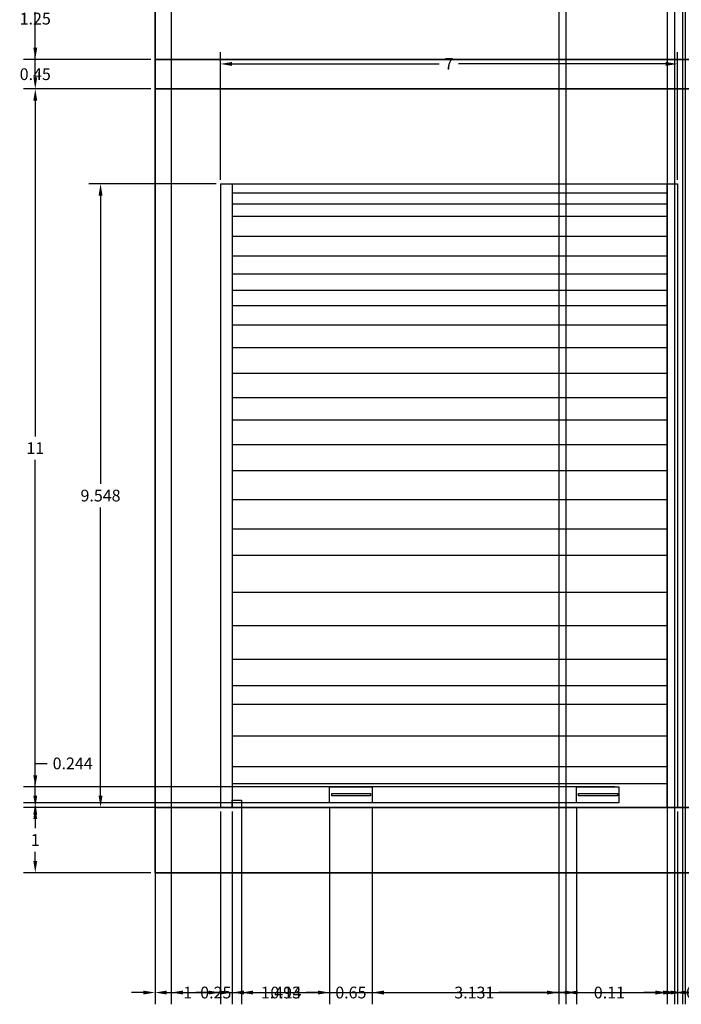
# Model space of a CAD drawing. Units: millimetres. Extents: x 2473 to 2512.3, y 2191.3 to 2230.4.
# Tile 1 of 8: x 2473.5 to 2483.7, y 2191.3 to 2206.4. Entities that reach past the tile are written whole.
import ezdxf

# ---------------------------------------------------------------- set-up
doc = ezdxf.new("R2010")
doc.units = ezdxf.units.MM
for name, color, linetype, lineweight in [('A-ANNO-DIMS', 2, 'Continuous', 18), ('A-DOOR', 4, 'Continuous', 25), ('A-ELEV', 7, 'Continuous', 35)]:
    doc.layers.add(name, color=color, linetype=linetype, lineweight=lineweight)
doc.styles.get("Standard").update_dxf_attribs({"font": 'arial.ttf'})
doc.dimstyles.get("Standard").update_dxf_attribs({"dimtxt": 0.18, "dimasz": 0.18, "dimexe": 0.18, "dimexo": 0.0625, "dimgap": 0.09, "dimtad": 0, "dimtih": 1, "dimtoh": 1, "dimdec": 4, "dimzin": 0, "dimdsep": 46, "dimtxsty": 'Standard', "dimcen": 0.09, "dimadec": 0, "dimazin": 0, "dimtfac": 1, "dimtdec": 4, "dimtofl": 0, "dimtmove": 0, "dimatfit": 3, "dimfxl": 1, "dimtolj": 1, "dimtzin": 0, "dimarcsym": 0})

# ---------------------------------------------------------------- blocks, each defined once
blk = doc.blocks.new('*D7')
at = {"layer": 'A-ANNO-DIMS', "color": 0, "lineweight": -2, "transparency": 16777216}
for p, q in [((2475.623, 2193.292), (2475.623, 2191.34)), ((2507.623, 2193.292), (2507.623, 2191.34)), ((2475.803, 2191.52), (2491.405, 2191.52)), ((2507.443, 2191.52), (2491.841, 2191.52))]:
    blk.add_line(p, q, dxfattribs=at)
at = {"layer": 'A-ANNO-DIMS', "color": 0, "transparency": 16777216}
for points in [[(2475.803, 2191.55), (2475.803, 2191.49), (2475.623, 2191.52)], [(2507.443, 2191.55), (2507.443, 2191.49), (2507.623, 2191.52)]]:
    blk.add_solid(points, dxfattribs=at)
at = {"layer": 'Defpoints', "color": 0, "transparency": 16777216}
for p in [(2475.623, 2193.355), (2507.623, 2193.355), (2507.623, 2191.52)]:
    blk.add_point(p, dxfattribs=at)
at = {"layer": 'A-ANNO-DIMS', "color": 0, "transparency": 16777216, "insert": (2491.623, 2191.52), "char_height": 0.18, "attachment_point": 5}
blk.add_mtext('\\A1;32', dxfattribs=at)
blk = doc.blocks.new('*D10')
at = {"layer": 'A-ANNO-DIMS', "color": 0, "lineweight": -2, "transparency": 16777216}
for p, q in [((2475.56, 2194.355), (2473.608, 2194.355)), ((2473.788, 2194.175), (2473.788, 2194.035)), ((2473.788, 2193.535), (2473.788, 2193.675)), ((2475.56, 2193.355), (2473.608, 2193.355))]:
    blk.add_line(p, q, dxfattribs=at)
at = {"layer": 'A-ANNO-DIMS', "color": 0, "transparency": 16777216}
for points in [[(2473.758, 2194.175), (2473.818, 2194.175), (2473.788, 2194.355)], [(2473.758, 2193.535), (2473.818, 2193.535), (2473.788, 2193.355)]]:
    blk.add_solid(points, dxfattribs=at)
at = {"layer": 'Defpoints', "color": 0, "transparency": 16777216}
for p in [(2473.788, 2194.355), (2475.623, 2194.355), (2475.623, 2193.355)]:
    blk.add_point(p, dxfattribs=at)
at = {"layer": 'A-ANNO-DIMS', "color": 0, "transparency": 16777216, "insert": (2473.788, 2193.855), "char_height": 0.18, "attachment_point": 5}
blk.add_mtext('\\A1;1', dxfattribs=at)
blk = doc.blocks.new('*D11')
at = {"layer": 'A-ANNO-DIMS', "color": 0, "lineweight": -2, "transparency": 16777216}
for p, q in [((2475.56, 2205.355), (2473.608, 2205.355)), ((2473.788, 2205.175), (2473.788, 2200.035)), ((2473.788, 2194.535), (2473.788, 2199.675)), ((2475.56, 2194.355), (2473.608, 2194.355))]:
    blk.add_line(p, q, dxfattribs=at)
at = {"layer": 'A-ANNO-DIMS', "color": 0, "transparency": 16777216}
for points in [[(2473.758, 2205.175), (2473.818, 2205.175), (2473.788, 2205.355)], [(2473.758, 2194.535), (2473.818, 2194.535), (2473.788, 2194.355)]]:
    blk.add_solid(points, dxfattribs=at)
at = {"layer": 'Defpoints', "color": 0, "transparency": 16777216}
for p in [(2473.788, 2205.355), (2475.623, 2205.355), (2475.623, 2194.355)]:
    blk.add_point(p, dxfattribs=at)
at = {"layer": 'A-ANNO-DIMS', "color": 0, "transparency": 16777216, "insert": (2473.788, 2199.855), "char_height": 0.18, "attachment_point": 5}
blk.add_mtext('\\A1;11', dxfattribs=at)
blk = doc.blocks.new('*D12')
at = {"layer": 'A-ANNO-DIMS', "color": 0, "lineweight": -2, "transparency": 16777216}
for p, q in [((2475.56, 2219.055), (2473.608, 2219.055)), ((2473.788, 2218.875), (2473.788, 2212.387)), ((2473.788, 2205.535), (2473.788, 2212.023)), ((2475.56, 2205.355), (2473.608, 2205.355))]:
    blk.add_line(p, q, dxfattribs=at)
at = {"layer": 'A-ANNO-DIMS', "color": 0, "transparency": 16777216}
for points in [[(2473.758, 2218.875), (2473.818, 2218.875), (2473.788, 2219.055)], [(2473.758, 2205.535), (2473.818, 2205.535), (2473.788, 2205.355)]]:
    blk.add_solid(points, dxfattribs=at)
at = {"layer": 'Defpoints', "color": 0, "transparency": 16777216}
for p in [(2473.788, 2219.055), (2475.623, 2219.055), (2475.623, 2205.355)]:
    blk.add_point(p, dxfattribs=at)
at = {"layer": 'A-ANNO-DIMS', "color": 0, "transparency": 16777216, "insert": (2473.788, 2212.205), "char_height": 0.18, "attachment_point": 5}
blk.add_mtext('\\A1;13.7', dxfattribs=at)
blk = doc.blocks.new('*D14')
at = {"layer": 'A-ANNO-DIMS', "color": 0, "lineweight": -2, "transparency": 16777216}
for p, q in [((2476.623, 2203.965), (2476.623, 2205.918)), ((2483.623, 2203.965), (2483.623, 2205.918)), ((2476.803, 2205.738), (2479.975, 2205.738)), ((2483.443, 2205.738), (2480.271, 2205.738))]:
    blk.add_line(p, q, dxfattribs=at)
at = {"layer": 'A-ANNO-DIMS', "color": 0, "transparency": 16777216}
for points in [[(2476.803, 2205.768), (2476.803, 2205.708), (2476.623, 2205.738)], [(2483.443, 2205.768), (2483.443, 2205.708), (2483.623, 2205.738)]]:
    blk.add_solid(points, dxfattribs=at)
at = {"layer": 'Defpoints', "color": 0, "transparency": 16777216}
for p in [(2483.623, 2205.738), (2476.623, 2203.903), (2483.623, 2203.903)]:
    blk.add_point(p, dxfattribs=at)
at = {"layer": 'A-ANNO-DIMS', "color": 0, "transparency": 16777216, "insert": (2480.123, 2205.738), "char_height": 0.18, "attachment_point": 5}
blk.add_mtext('\\A1;7', dxfattribs=at)
blk = doc.blocks.new('*D17')
at = {"layer": 'A-ANNO-DIMS', "color": 0, "lineweight": -2, "transparency": 16777216}
for p, q in [((2476.56, 2203.903), (2474.608, 2203.903)), ((2474.788, 2203.723), (2474.788, 2199.311)), ((2474.788, 2194.535), (2474.788, 2198.947)), ((2476.56, 2194.355), (2474.608, 2194.355))]:
    blk.add_line(p, q, dxfattribs=at)
at = {"layer": 'A-ANNO-DIMS', "color": 0, "transparency": 16777216}
for points in [[(2474.758, 2203.723), (2474.818, 2203.723), (2474.788, 2203.903)], [(2474.758, 2194.535), (2474.818, 2194.535), (2474.788, 2194.355)]]:
    blk.add_solid(points, dxfattribs=at)
at = {"layer": 'Defpoints', "color": 0, "transparency": 16777216}
for p in [(2474.788, 2203.903), (2476.623, 2203.903), (2476.623, 2194.355)]:
    blk.add_point(p, dxfattribs=at)
at = {"layer": 'A-ANNO-DIMS', "color": 0, "transparency": 16777216, "insert": (2474.788, 2199.129), "char_height": 0.18, "attachment_point": 5}
blk.add_mtext('\\A1;9.548', dxfattribs=at)
blk = doc.blocks.new('*D23')
at = {"layer": 'A-ANNO-DIMS', "color": 0, "lineweight": -2, "transparency": 16777216}
for p, q in [((2475.623, 2194.292), (2475.623, 2191.34)), ((2476.623, 2194.292), (2476.623, 2191.34)), ((2475.803, 2191.52), (2476, 2191.52)), ((2476.443, 2191.52), (2476.246, 2191.52))]:
    blk.add_line(p, q, dxfattribs=at)
at = {"layer": 'A-ANNO-DIMS', "color": 0, "transparency": 16777216}
for points in [[(2475.803, 2191.55), (2475.803, 2191.49), (2475.623, 2191.52)], [(2476.443, 2191.55), (2476.443, 2191.49), (2476.623, 2191.52)]]:
    blk.add_solid(points, dxfattribs=at)
at = {"layer": 'Defpoints', "color": 0, "transparency": 16777216}
for p in [(2475.623, 2194.355), (2476.623, 2194.355), (2476.623, 2191.52)]:
    blk.add_point(p, dxfattribs=at)
at = {"layer": 'A-ANNO-DIMS', "color": 0, "transparency": 16777216, "insert": (2476.123, 2191.52), "char_height": 0.18, "attachment_point": 5}
blk.add_mtext('\\A1;1', dxfattribs=at)
blk = doc.blocks.new('*D24')
at = {"layer": 'A-ANNO-DIMS', "color": 0, "lineweight": -2, "transparency": 16777216}
for p, q in [((2483.623, 2194.292), (2483.623, 2191.34)), ((2484.37, 2194.292), (2484.37, 2191.34)), ((2483.443, 2191.52), (2483.263, 2191.52)), ((2484.55, 2191.52), (2484.73, 2191.52))]:
    blk.add_line(p, q, dxfattribs=at)
at = {"layer": 'A-ANNO-DIMS', "color": 0, "transparency": 16777216}
for points in [[(2483.443, 2191.55), (2483.443, 2191.49), (2483.623, 2191.52)], [(2484.55, 2191.55), (2484.55, 2191.49), (2484.37, 2191.52)]]:
    blk.add_solid(points, dxfattribs=at)
at = {"layer": 'Defpoints', "color": 0, "transparency": 16777216}
for p in [(2483.623, 2194.355), (2484.37, 2194.355), (2484.37, 2191.52)]:
    blk.add_point(p, dxfattribs=at)
at = {"layer": 'A-ANNO-DIMS', "color": 0, "transparency": 16777216, "insert": (2483.996, 2191.52), "char_height": 0.18, "attachment_point": 5}
blk.add_mtext('\\A1;0.75', dxfattribs=at)
blk = doc.blocks.new('*D37')
at = {"layer": 'A-ANNO-DIMS', "color": 0, "lineweight": -2, "transparency": 16777216}
for p, q in [((2473.788, 2205.988), (2473.788, 2206.168)), ((2475.56, 2205.808), (2473.608, 2205.808)), ((2475.56, 2205.355), (2473.608, 2205.355)), ((2473.788, 2205.175), (2473.788, 2204.995))]:
    blk.add_line(p, q, dxfattribs=at)
at = {"layer": 'A-ANNO-DIMS', "color": 0, "transparency": 16777216}
for points in [[(2473.758, 2205.988), (2473.818, 2205.988), (2473.788, 2205.808)], [(2473.758, 2205.175), (2473.818, 2205.175), (2473.788, 2205.355)]]:
    blk.add_solid(points, dxfattribs=at)
at = {"layer": 'Defpoints', "color": 0, "transparency": 16777216}
for p in [(2473.788, 2205.808), (2475.623, 2205.808), (2475.623, 2205.355)]:
    blk.add_point(p, dxfattribs=at)
at = {"layer": 'A-ANNO-DIMS', "color": 0, "transparency": 16777216, "insert": (2473.788, 2205.581), "char_height": 0.18, "attachment_point": 5}
blk.add_mtext('\\A1;0.45', dxfattribs=at)
blk = doc.blocks.new('*D38')
at = {"layer": 'A-ANNO-DIMS', "color": 0, "lineweight": -2, "transparency": 16777216}
for p, q in [((2476.56, 2207.055), (2473.608, 2207.055)), ((2473.788, 2206.875), (2473.788, 2206.613)), ((2473.788, 2205.988), (2473.788, 2206.249)), ((2475.56, 2205.808), (2473.608, 2205.808))]:
    blk.add_line(p, q, dxfattribs=at)
at = {"layer": 'A-ANNO-DIMS', "color": 0, "transparency": 16777216}
for points in [[(2473.758, 2206.875), (2473.818, 2206.875), (2473.788, 2207.055)], [(2473.758, 2205.988), (2473.818, 2205.988), (2473.788, 2205.808)]]:
    blk.add_solid(points, dxfattribs=at)
at = {"layer": 'Defpoints', "color": 0, "transparency": 16777216}
for p in [(2473.788, 2207.055), (2476.623, 2207.055), (2475.623, 2205.808)]:
    blk.add_point(p, dxfattribs=at)
at = {"layer": 'A-ANNO-DIMS', "color": 0, "transparency": 16777216, "insert": (2473.788, 2206.431), "char_height": 0.18, "attachment_point": 5}
blk.add_mtext('\\A1;1.25', dxfattribs=at)
blk = doc.blocks.new('*D93')
at = {"layer": 'A-ANNO-DIMS', "color": 0, "lineweight": -2, "transparency": 16777216}
for p, q in [((2476.804, 2194.292), (2476.804, 2191.34)), ((2478.297, 2194.362), (2478.297, 2191.34)), ((2476.984, 2191.52), (2477.165, 2191.52)), ((2478.117, 2191.52), (2477.935, 2191.52))]:
    blk.add_line(p, q, dxfattribs=at)
at = {"layer": 'A-ANNO-DIMS', "color": 0, "transparency": 16777216}
for points in [[(2476.984, 2191.55), (2476.984, 2191.49), (2476.804, 2191.52)], [(2478.117, 2191.55), (2478.117, 2191.49), (2478.297, 2191.52)]]:
    blk.add_solid(points, dxfattribs=at)
at = {"layer": 'Defpoints', "color": 0, "transparency": 16777216}
for p in [(2478.297, 2194.424), (2476.804, 2194.355), (2478.297, 2191.52)]:
    blk.add_point(p, dxfattribs=at)
at = {"layer": 'A-ANNO-DIMS', "color": 0, "transparency": 16777216, "insert": (2477.55, 2191.52), "char_height": 0.18, "attachment_point": 5}
blk.add_mtext('\\A1;1.493', dxfattribs=at)
blk = doc.blocks.new('*D94')
at = {"layer": 'A-ANNO-DIMS', "color": 0, "lineweight": -2, "transparency": 16777216}
for p, q in [((2478.297, 2194.362), (2478.297, 2191.34)), ((2478.947, 2194.362), (2478.947, 2191.34)), ((2478.117, 2191.52), (2477.937, 2191.52)), ((2479.127, 2191.52), (2479.307, 2191.52))]:
    blk.add_line(p, q, dxfattribs=at)
at = {"layer": 'A-ANNO-DIMS', "color": 0, "transparency": 16777216}
for points in [[(2478.117, 2191.55), (2478.117, 2191.49), (2478.297, 2191.52)], [(2479.127, 2191.55), (2479.127, 2191.49), (2478.947, 2191.52)]]:
    blk.add_solid(points, dxfattribs=at)
at = {"layer": 'Defpoints', "color": 0, "transparency": 16777216}
for p in [(2478.297, 2194.424), (2478.947, 2194.424), (2478.947, 2191.52)]:
    blk.add_point(p, dxfattribs=at)
at = {"layer": 'A-ANNO-DIMS', "color": 0, "transparency": 16777216, "insert": (2478.622, 2191.52), "char_height": 0.18, "attachment_point": 5}
blk.add_mtext('\\A1;0.65', dxfattribs=at)
blk = doc.blocks.new('*D95')
at = {"layer": 'A-ANNO-DIMS', "color": 0, "lineweight": -2, "transparency": 16777216}
for p, q in [((2478.947, 2194.362), (2478.947, 2191.34)), ((2482.078, 2194.362), (2482.078, 2191.34)), ((2479.127, 2191.52), (2480.136, 2191.52)), ((2481.898, 2191.52), (2480.889, 2191.52))]:
    blk.add_line(p, q, dxfattribs=at)
at = {"layer": 'A-ANNO-DIMS', "color": 0, "transparency": 16777216}
for points in [[(2479.127, 2191.55), (2479.127, 2191.49), (2478.947, 2191.52)], [(2481.898, 2191.55), (2481.898, 2191.49), (2482.078, 2191.52)]]:
    blk.add_solid(points, dxfattribs=at)
at = {"layer": 'Defpoints', "color": 0, "transparency": 16777216}
for p in [(2478.947, 2194.424), (2482.078, 2194.424), (2482.078, 2191.52)]:
    blk.add_point(p, dxfattribs=at)
at = {"layer": 'A-ANNO-DIMS', "color": 0, "transparency": 16777216, "insert": (2480.513, 2191.52), "char_height": 0.18, "attachment_point": 5}
blk.add_mtext('\\A1;3.131', dxfattribs=at)
blk = doc.blocks.new('*D96')
at = {"layer": 'A-ANNO-DIMS', "color": 0, "lineweight": -2, "transparency": 16777216}
for p, q in [((2473.788, 2194.848), (2473.788, 2195.028)), ((2473.788, 2195.028), (2473.968, 2195.028)), ((2482.666, 2194.668), (2473.608, 2194.668)), ((2482.666, 2194.424), (2473.608, 2194.424)), ((2473.788, 2194.244), (2473.788, 2194.064))]:
    blk.add_line(p, q, dxfattribs=at)
at = {"layer": 'A-ANNO-DIMS', "color": 0, "transparency": 16777216}
for points in [[(2473.758, 2194.848), (2473.818, 2194.848), (2473.788, 2194.668)], [(2473.758, 2194.244), (2473.818, 2194.244), (2473.788, 2194.424)]]:
    blk.add_solid(points, dxfattribs=at)
at = {"layer": 'Defpoints', "color": 0, "transparency": 16777216}
for p in [(2473.788, 2194.668), (2482.729, 2194.668), (2482.729, 2194.424)]:
    blk.add_point(p, dxfattribs=at)
at = {"layer": 'A-ANNO-DIMS', "color": 0, "transparency": 16777216, "insert": (2474.361, 2195.028), "char_height": 0.18, "attachment_point": 5}
blk.add_mtext('\\A1;0.244', dxfattribs=at)
blk = doc.blocks.new('*D98')
at = {"layer": 'A-ANNO-DIMS', "color": 0, "lineweight": -2, "transparency": 16777216}
for p, q in [((2476.945, 2194.402), (2476.945, 2191.34)), ((2476.804, 2194.292), (2476.804, 2191.34)), ((2476.624, 2191.52), (2476.444, 2191.52)), ((2477.125, 2191.52), (2477.305, 2191.52))]:
    blk.add_line(p, q, dxfattribs=at)
at = {"layer": 'A-ANNO-DIMS', "color": 0, "transparency": 16777216}
for points in [[(2476.624, 2191.55), (2476.624, 2191.49), (2476.804, 2191.52)], [(2477.125, 2191.55), (2477.125, 2191.49), (2476.945, 2191.52)]]:
    blk.add_solid(points, dxfattribs=at)
at = {"layer": 'Defpoints', "color": 0, "transparency": 16777216}
for p in [(2476.945, 2194.464), (2476.804, 2194.355), (2476.945, 2191.52)]:
    blk.add_point(p, dxfattribs=at)
at = {"layer": 'A-ANNO-DIMS', "color": 0, "transparency": 16777216, "insert": (2477.628, 2191.52), "char_height": 0.18, "attachment_point": 5}
blk.add_mtext('\\A1;0.14', dxfattribs=at)
blk = doc.blocks.new('*D102')
at = {"layer": 'A-ANNO-DIMS', "color": 0, "lineweight": -2, "transparency": 16777216}
for p, q in [((2483.468, 2209.664), (2483.468, 2191.34)), ((2483.581, 2209.664), (2483.581, 2191.34)), ((2483.288, 2191.52), (2483.108, 2191.52)), ((2483.761, 2191.52), (2483.941, 2191.52))]:
    blk.add_line(p, q, dxfattribs=at)
at = {"layer": 'A-ANNO-DIMS', "color": 0, "transparency": 16777216}
for points in [[(2483.288, 2191.55), (2483.288, 2191.49), (2483.468, 2191.52)], [(2483.761, 2191.55), (2483.761, 2191.49), (2483.581, 2191.52)]]:
    blk.add_solid(points, dxfattribs=at)
at = {"layer": 'Defpoints', "color": 0, "transparency": 16777216}
for p in [(2483.468, 2209.727), (2483.581, 2209.727), (2483.581, 2191.52)]:
    blk.add_point(p, dxfattribs=at)
at = {"layer": 'A-ANNO-DIMS', "color": 0, "transparency": 16777216, "insert": (2484.248, 2191.52), "char_height": 0.18, "attachment_point": 5}
blk.add_mtext('\\A1;0.11', dxfattribs=at)
blk = doc.blocks.new('*D103')
at = {"layer": 'A-ANNO-DIMS', "color": 0, "lineweight": -2, "transparency": 16777216}
for p, q in [((2483.581, 2209.664), (2483.581, 2191.34)), ((2483.702, 2209.684), (2483.702, 2191.34)), ((2483.401, 2191.52), (2483.221, 2191.52)), ((2483.882, 2191.52), (2484.062, 2191.52))]:
    blk.add_line(p, q, dxfattribs=at)
at = {"layer": 'A-ANNO-DIMS', "color": 0, "transparency": 16777216}
for points in [[(2483.401, 2191.55), (2483.401, 2191.49), (2483.581, 2191.52)], [(2483.882, 2191.55), (2483.882, 2191.49), (2483.702, 2191.52)]]:
    blk.add_solid(points, dxfattribs=at)
at = {"layer": 'Defpoints', "color": 0, "transparency": 16777216}
for p in [(2483.581, 2209.727), (2483.702, 2209.747), (2483.702, 2191.52)]:
    blk.add_point(p, dxfattribs=at)
at = {"layer": 'A-ANNO-DIMS', "color": 0, "transparency": 16777216, "insert": (2484.439, 2191.52), "char_height": 0.18, "attachment_point": 5}
blk.add_mtext('\\A1;0.121', dxfattribs=at)
blk = doc.blocks.new('*D104')
at = {"layer": 'A-ANNO-DIMS', "color": 0, "lineweight": -2, "transparency": 16777216}
for p, q in [((2483.702, 2209.684), (2483.702, 2191.34)), ((2483.744, 2209.684), (2483.744, 2191.34)), ((2483.522, 2191.52), (2483.342, 2191.52)), ((2483.924, 2191.52), (2484.104, 2191.52))]:
    blk.add_line(p, q, dxfattribs=at)
at = {"layer": 'A-ANNO-DIMS', "color": 0, "transparency": 16777216}
for points in [[(2483.522, 2191.55), (2483.522, 2191.49), (2483.702, 2191.52)], [(2483.924, 2191.55), (2483.924, 2191.49), (2483.744, 2191.52)]]:
    blk.add_solid(points, dxfattribs=at)
at = {"layer": 'Defpoints', "color": 0, "transparency": 16777216}
for p in [(2483.702, 2209.747), (2483.744, 2209.747), (2483.744, 2191.52)]:
    blk.add_point(p, dxfattribs=at)
at = {"layer": 'A-ANNO-DIMS', "color": 0, "transparency": 16777216, "insert": (2484.497, 2191.52), "char_height": 0.18, "attachment_point": 5}
blk.add_mtext('\\A1;0.042', dxfattribs=at)
blk = doc.blocks.new('*D126')
at = {"layer": 'A-ANNO-DIMS', "color": 0, "lineweight": -2, "transparency": 16777216}
for p, q in [((2475.869, 2223.101), (2475.869, 2191.34)), ((2475.623, 2222.992), (2475.623, 2191.34)), ((2475.443, 2191.52), (2475.263, 2191.52)), ((2476.049, 2191.52), (2476.229, 2191.52))]:
    blk.add_line(p, q, dxfattribs=at)
at = {"layer": 'A-ANNO-DIMS', "color": 0, "transparency": 16777216}
for points in [[(2475.443, 2191.55), (2475.443, 2191.49), (2475.623, 2191.52)], [(2476.049, 2191.55), (2476.049, 2191.49), (2475.869, 2191.52)]]:
    blk.add_solid(points, dxfattribs=at)
at = {"layer": 'Defpoints', "color": 0, "transparency": 16777216}
for p in [(2475.623, 2223.055), (2475.869, 2223.163), (2475.869, 2191.52)]:
    blk.add_point(p, dxfattribs=at)
at = {"layer": 'A-ANNO-DIMS', "color": 0, "transparency": 16777216, "insert": (2476.553, 2191.52), "char_height": 0.18, "attachment_point": 5}
blk.add_mtext('\\A1;0.25', dxfattribs=at)
blk = doc.blocks.new('*D129')
at = {"layer": 'A-ANNO-DIMS', "color": 0, "lineweight": -2, "transparency": 16777216}
for p, q in [((2481.806, 2223.101), (2481.806, 2191.34)), ((2481.915, 2222.992), (2481.915, 2191.34)), ((2481.626, 2191.52), (2481.446, 2191.52)), ((2482.095, 2191.52), (2482.275, 2191.52))]:
    blk.add_line(p, q, dxfattribs=at)
at = {"layer": 'A-ANNO-DIMS', "color": 0, "transparency": 16777216}
for points in [[(2481.626, 2191.55), (2481.626, 2191.49), (2481.806, 2191.52)], [(2482.095, 2191.55), (2482.095, 2191.49), (2481.915, 2191.52)]]:
    blk.add_solid(points, dxfattribs=at)
at = {"layer": 'Defpoints', "color": 0, "transparency": 16777216}
for p in [(2481.806, 2223.163), (2481.915, 2223.055), (2481.915, 2191.52)]:
    blk.add_point(p, dxfattribs=at)
at = {"layer": 'A-ANNO-DIMS', "color": 0, "transparency": 16777216, "insert": (2482.582, 2191.52), "char_height": 0.18, "attachment_point": 5}
blk.add_mtext('\\A1;0.11', dxfattribs=at)

msp = doc.modelspace()

# ---------------------------------------------------------------- linework, layer by layer
at = {"layer": 'A-DOOR'}
for p, q in [((2476.6229, 2203.9027), (2483.6229, 2203.9027)), ((2476.6229, 2203.9027), (2476.6229, 2194.3549)), ((2476.8036, 2203.9027), (2476.8036, 2194.3549)), ((2483.464, 2203.9027), (2483.464, 2194.3549)), ((2483.6229, 2203.9027), (2483.6229, 2194.3549)), ((2476.8036, 2203.7647), (2483.464, 2203.7647)), ((2476.8036, 2203.5963), (2483.464, 2203.5963)), ((2476.8036, 2203.4067), (2483.464, 2203.4067)), ((2476.8036, 2203.1), (2483.464, 2203.1)), ((2476.8036, 2202.7988), (2483.464, 2202.7988)), ((2476.8036, 2202.5255), (2483.464, 2202.5255)), ((2476.8036, 2202.2745), (2483.464, 2202.2745)), ((2476.8036, 2202.0402), (2483.464, 2202.0402)), ((2476.8036, 2201.7408), (2483.464, 2201.7408)), ((2476.8036, 2201.3981), (2483.464, 2201.3981)), ((2476.8036, 2201.0013), (2483.464, 2201.0013)), ((2476.8036, 2200.6315), (2483.464, 2200.6315)), ((2476.8036, 2200.2888), (2483.464, 2200.2888)), ((2476.8036, 2199.91), (2483.464, 2199.91)), ((2476.8036, 2199.5132), (2483.464, 2199.5132)), ((2476.8036, 2199.0712), (2483.464, 2199.0712)), ((2476.8036, 2198.621), (2483.464, 2198.621)), ((2476.8036, 2198.218), (2483.464, 2198.218)), ((2476.8036, 2197.6503), (2483.464, 2197.6503)), ((2476.8036, 2197.1375), (2483.464, 2197.1375)), ((2476.8036, 2196.6247), (2483.464, 2196.6247)), ((2476.8036, 2196.2209), (2483.464, 2196.2209)), ((2476.8036, 2195.9338), (2483.464, 2195.9338)), ((2476.8036, 2195.4522), (2483.464, 2195.4522)), ((2476.8036, 2194.9798), (2483.464, 2194.9798)), ((2476.8036, 2194.7229), (2483.464, 2194.7229))]:
    msp.add_line(p, q, dxfattribs=at)
for points in [[(2478.2966, 2194.6682), (2478.9472, 2194.6682), (2478.9472, 2194.4242), (2478.2966, 2194.4242)], [(2478.3295, 2194.5673), (2478.9239, 2194.5673), (2478.9239, 2194.5329), (2478.3295, 2194.5329)], [(2482.0783, 2194.6682), (2482.7289, 2194.6682), (2482.7289, 2194.4242), (2482.0783, 2194.4242)], [(2482.1112, 2194.5673), (2482.7056, 2194.5673), (2482.7056, 2194.5329), (2482.1112, 2194.5329)], [(2476.8036, 2194.4642), (2476.9451, 2194.4642), (2476.9451, 2194.3549), (2476.8036, 2194.3549)]]:
    msp.add_lwpolyline(points, close=True, dxfattribs=at)
at = {"layer": 'A-ELEV'}
for p, q in [((2475.6229, 2193.3549), (2475.6229, 2219.0549)), ((2507.6229, 2205.8077), (2475.6229, 2205.8077)), ((2507.6229, 2205.3549), (2475.6229, 2205.3549)), ((2491.6229, 2194.3549), (2475.6229, 2194.3549)), ((2507.6229, 2193.3549), (2475.6229, 2193.3549))]:
    msp.add_line(p, q, dxfattribs=at)

# ---------------------------------------------------------------- dimensions: what is measured, and where the dimension line sits
at = {"layer": 'A-ANNO-DIMS'}
for base, p1, p2, override, picture, middle in [((2475.869, 2191.5199), (2475.6229, 2223.0549), (2475.869, 2223.1632), {"dimdec": 2, "dimlfac": 1, "dimrnd": 0, "dimzin": 0, "dimdsep": 46, "dimlunit": 2}, '*D126', (2476.5535, 2191.5199)), ((2481.9154, 2191.5199), (2481.806, 2223.1632), (2481.9154, 2223.0549), {"dimdec": 2, "dimlfac": 1, "dimrnd": 0, "dimzin": 0, "dimdsep": 46, "dimlunit": 2}, '*D129', (2482.5818, 2191.5199)), ((2483.5812, 2191.5199), (2483.4683, 2209.7269), (2483.5812, 2209.7269), {"dimdec": 2, "dimlfac": 1, "dimrnd": 0, "dimzin": 0, "dimdsep": 46, "dimlunit": 2}, '*D102', (2484.2476, 2191.5199)), ((2483.7022, 2191.5199), (2483.5812, 2209.7269), (2483.7022, 2209.7466), {"dimdec": 3, "dimlfac": 1, "dimrnd": 0, "dimzin": 0, "dimdsep": 46, "dimlunit": 2}, '*D103', (2484.4385, 2191.5199)), ((2483.7441, 2191.5199), (2483.7022, 2209.7466), (2483.7441, 2209.7466), {"dimdec": 3, "dimlfac": 1, "dimrnd": 0, "dimzin": 0, "dimdsep": 46, "dimlunit": 2}, '*D104', (2484.4969, 2191.5199)), ((2483.6229, 2205.7377), (2476.6229, 2203.9027), (2483.6229, 2203.9027), {"dimdec": 0, "dimlfac": 1, "dimrnd": 0, "dimzin": 0, "dimdsep": 46, "dimlunit": 2}, '*D14', (2480.1229, 2205.7377)), ((2476.9451, 2191.5199), (2476.8036, 2194.3549), (2476.9451, 2194.4642), {"dimdec": 2, "dimlfac": 1, "dimrnd": 0, "dimzin": 0, "dimdsep": 46, "dimlunit": 2}, '*D98', (2477.6285, 2191.5199)), ((2478.2966, 2191.5199), (2476.8036, 2194.3549), (2478.2966, 2194.4242), {"dimdec": 3, "dimlfac": 1, "dimrnd": 0, "dimzin": 0, "dimdsep": 46, "dimlunit": 2}, '*D93', (2477.5501, 2191.5199)), ((2478.9472, 2191.5199), (2478.2966, 2194.4242), (2478.9472, 2194.4242), {"dimdec": 2, "dimlfac": 1, "dimrnd": 0, "dimzin": 0, "dimdsep": 46, "dimlunit": 2}, '*D94', (2478.6219, 2191.5199)), ((2482.0783, 2191.5199), (2478.9472, 2194.4242), (2482.0783, 2194.4242), {"dimdec": 3, "dimlfac": 1, "dimrnd": 0, "dimzin": 0, "dimdsep": 46, "dimlunit": 2}, '*D95', (2480.5127, 2191.5199)), ((2476.6229, 2191.5199), (2475.6229, 2194.3549), (2476.6229, 2194.3549), {"dimdec": 0, "dimlfac": 1, "dimrnd": 0, "dimzin": 0, "dimdsep": 46, "dimlunit": 2}, '*D23', (2476.1229, 2191.5199)), ((2484.3698, 2191.5199), (2483.6229, 2194.3549), (2484.3698, 2194.3549), {"dimdec": 2, "dimlfac": 1, "dimrnd": 0, "dimzin": 0, "dimdsep": 46, "dimlunit": 2}, '*D24', (2483.9963, 2191.5199)), ((2507.6229, 2191.5199), (2475.6229, 2193.3549), (2507.6229, 2193.3549), {"dimdec": 0, "dimlfac": 1, "dimrnd": 0, "dimzin": 0, "dimdsep": 46, "dimlunit": 2}, '*D7', (2491.6229, 2191.5199))]:
    dim = msp.add_linear_dim(base=base, p1=p1, p2=p2, dimstyle='Standard', override=override, dxfattribs=at)
    dim.commit()
    dim.dimension.update_dxf_attribs({"geometry": picture, "text_midpoint": middle})
for base, p1, p2, override, picture, middle in [((2473.7879, 2219.0549), (2475.6229, 2205.3549), (2475.6229, 2219.0549), {"dimdec": 1, "dimlfac": 1, "dimrnd": 0, "dimzin": 0, "dimdsep": 46, "dimlunit": 2}, '*D12', (2473.7879, 2212.2049)), ((2473.7879, 2207.0549), (2475.6229, 2205.8077), (2476.6229, 2207.0549), {"dimdec": 2, "dimlfac": 1, "dimrnd": 0, "dimzin": 0, "dimdsep": 46, "dimlunit": 2}, '*D38', (2473.7879, 2206.4313)), ((2473.7879, 2205.8077), (2475.6229, 2205.3549), (2475.6229, 2205.8077), {"dimdec": 2, "dimlfac": 1, "dimrnd": 0, "dimzin": 0, "dimdsep": 46, "dimlunit": 2}, '*D37', (2473.7879, 2205.5813)), ((2473.7879, 2205.3549), (2475.6229, 2194.3549), (2475.6229, 2205.3549), {"dimdec": 0, "dimlfac": 1, "dimrnd": 0, "dimzin": 0, "dimdsep": 46, "dimlunit": 2}, '*D11', (2473.7879, 2199.8549)), ((2474.7879, 2203.9027), (2476.6229, 2194.3549), (2476.6229, 2203.9027), {"dimdec": 3, "dimlfac": 1, "dimrnd": 0, "dimzin": 0, "dimdsep": 46, "dimlunit": 2}, '*D17', (2474.7879, 2199.1288)), ((2473.7879, 2194.6682), (2482.7289, 2194.4242), (2482.7289, 2194.6682), {"dimdec": 3, "dimlfac": 1, "dimrnd": 0, "dimzin": 0, "dimdsep": 46, "dimlunit": 2}, '*D96', (2474.3612, 2195.0282)), ((2473.7879, 2194.3549), (2475.6229, 2193.3549), (2475.6229, 2194.3549), {"dimdec": 0, "dimlfac": 1, "dimrnd": 0, "dimzin": 0, "dimdsep": 46, "dimlunit": 2}, '*D10', (2473.7879, 2193.8549))]:
    dim = msp.add_linear_dim(base=base, p1=p1, p2=p2, angle=90, dimstyle='Standard', override=override, dxfattribs=at)
    dim.commit()
    dim.dimension.update_dxf_attribs({"geometry": picture, "text_midpoint": middle})

doc.saveas('drawing.dxf')
